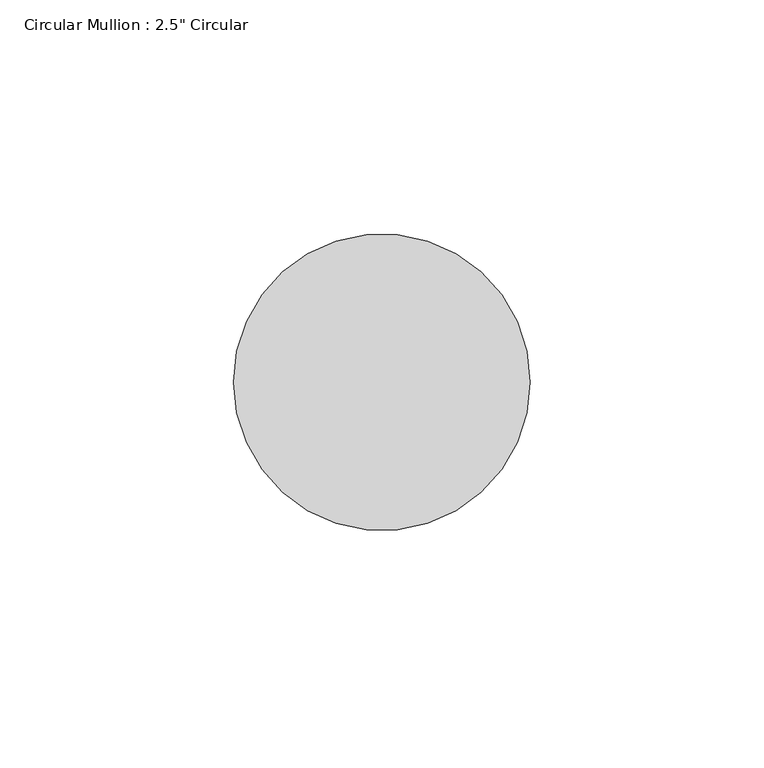
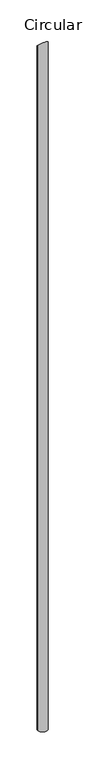
"""IFC4 building model written with IfcOpenShell, lengths in millimetres: member geometry."""

from ifc_helpers import new_model, si_unit, frame, origin, place, context, project, spatial, circle_curve, ellipse_curve, source, transform, mapped, element, save
from ifc_brep_helpers import plane_surface, cylinder_surface, advanced_brep


def member_2ad469c0(model_context):
    return source(origin(), model_context, "Body", "AdvancedBrep", [
        advanced_brep(
        [(0.0, 0.0, -4648.2), (-63.5, 0.0, -4648.2), (-63.5, 0.0, 0.0), (0.0, 0.0, 0.0)],
        [
            (0, 1, circle_curve(frame((-31.75, 0.0, -4648.2), z_axis=(0.0, 0.0, -1.0), x_axis=(1.0, 0.0, 0.0)), 31.75)),
            (1, 0, circle_curve(frame((-31.75, 0.0, -4648.2), z_axis=(0.0, 0.0, -1.0), x_axis=(1.0, 0.0, 0.0)), 31.75)),
            (2, 3, ellipse_curve(frame((-31.75, 0.0, 0.0), z_axis=(0.0, -0.707106781186547, -0.7071067811865481), x_axis=(0.0, -0.7071067811865481, 0.7071067811865468)), 44.9012806, 31.75)),
            (3, 0),
            (1, 2),
            (3, 2, ellipse_curve(frame((-31.75, 0.0, 0.0), z_axis=(0.0, -0.707106781186547, -0.7071067811865481), x_axis=(0.0, -0.7071067811865481, 0.7071067811865468)), 44.9012806, 31.75)),
        ],
        [
            plane_surface(frame((0.0, -63.5, -4648.2), z_axis=(0.0, 0.0, -1.0), x_axis=(-1.0, 0.0, 0.0))),
            cylinder_surface(frame((-31.75, 0.0, 0.0), z_axis=(0.0, 0.0, 1.0), x_axis=(1.0, 0.0, 0.0)), 31.75),
            plane_surface(frame((-304.8, 0.0, 0.0), z_axis=(0.0, 0.707106781186547, 0.7071067811865481), x_axis=(0.0, 0.7071067811865481, -0.707106781186547))),
        ],
        [
            (0, [[1, 2]]),
            (1, [[3, 4, -2, 5]]),
            (1, [[6, -5, -1, -4]]),
            (2, [[-3, -6]]),
        ],
    ),
    ])


if __name__ == "__main__":
    model = new_model("IFC4")
    model_context = context("Model", 3, world=origin())
    ifc_project = project(units=[si_unit("LENGTHUNIT", "METRE", prefix="MILLI")], contexts=[model_context])
    site = spatial("IfcSite", under=ifc_project)
    building = spatial("IfcBuilding", under=site)
    placement = place(None, origin())
    member_shape = member_2ad469c0(model_context)
    element("IfcMember", 1, ObjectType="Circular Mullion : 2.5\" Circular", at=placement, inside=building, context=model_context, shape_type="MappedRepresentation", body=[
        mapped(member_shape, transform((0.0, 0.0, 0.0), x_axis=(1.0, 0.0, 0.0), y_axis=(0.0, 1.0, 0.0), z_axis=(0.0, 0.0, 1.0))),
    ])
    save(model, "model.ifc")

# Revit data of these elements
# Type "Circular Mullion : 2.5\" Circular"
#   built-in parameter 1007350 = 0.104167 (stored number, unit not read)
# Element 1 (IfcMember, "Circular Mullion : 2.5\" Circular")
#   Materials on its faces: "Aluminum"
# Materials
#   "Aluminum": class "Metal", colour RGB 247 247 247, transparency 0, Description = "Aluminum 6061", Cost = 0
